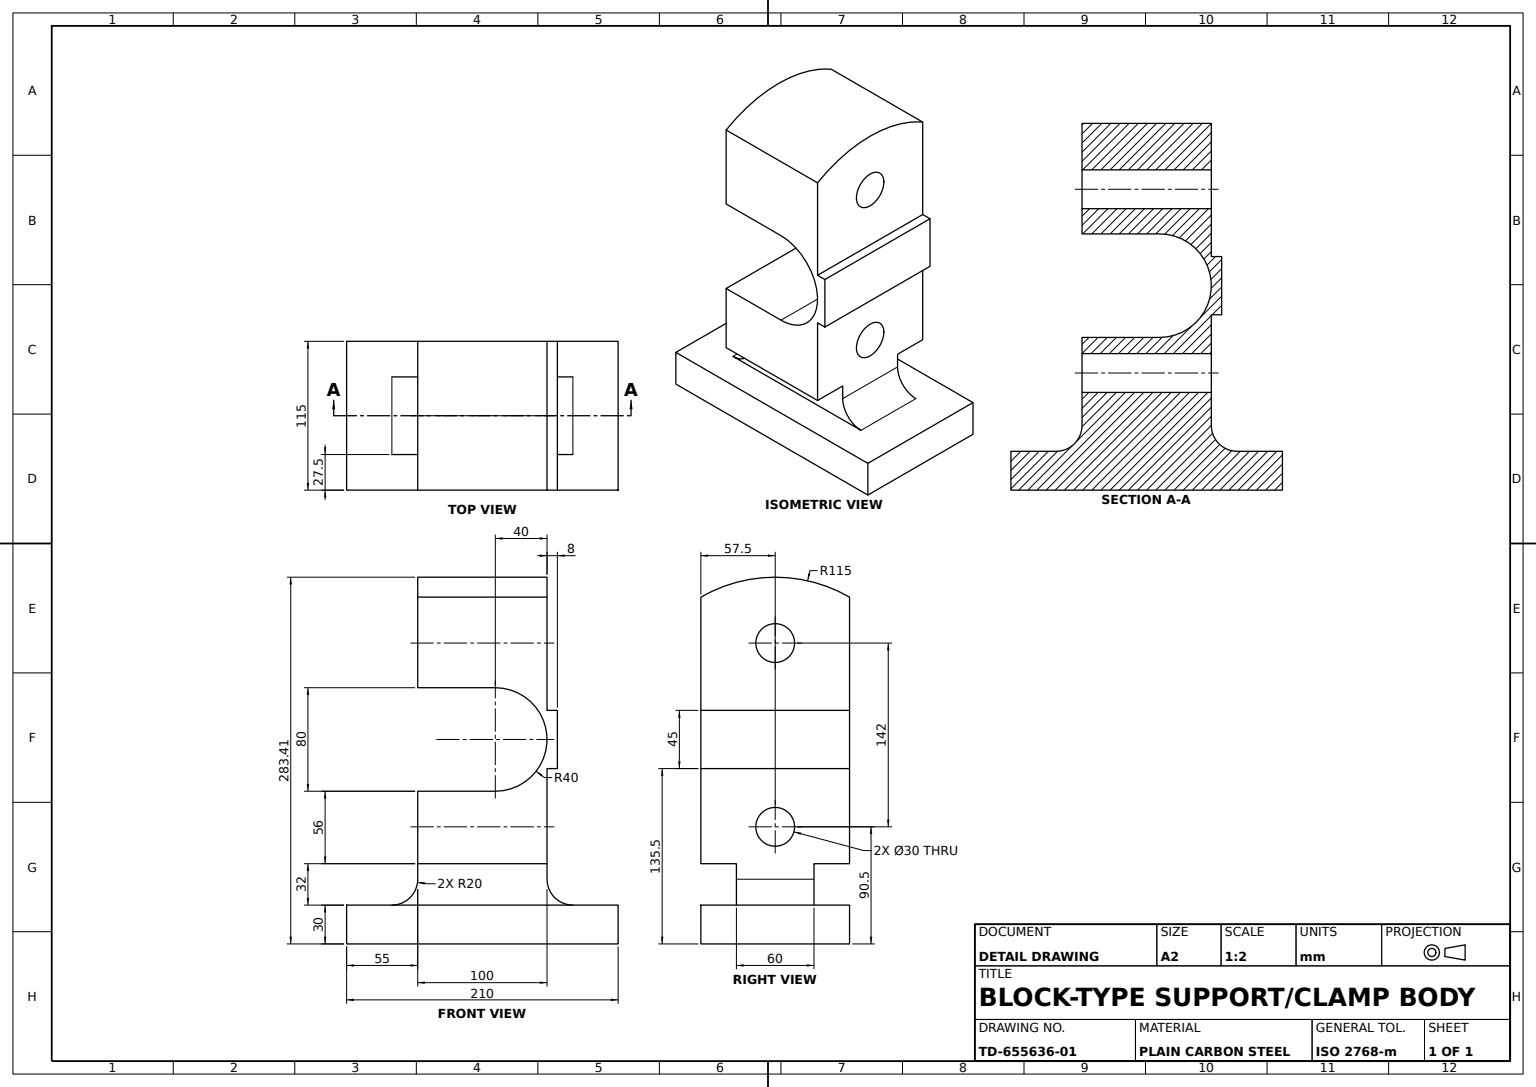
SolidWorks part; units mm, degrees
material "Plain Carbon Steel"
ref_plane "Front Plane" through (0, 0, 0) normal (0, 0, 1) x (1, 0, 0)
ref_plane "Top Plane" through (0, 0, 0) normal (0, 1, 0) x (1, 0, 0)
ref_plane "Right Plane" through (0, 0, 0) normal (1, 0, 0) x (0, 0, -1)
sketch "Base Plate Sketch" plane through (0, 0, 0) normal (0, 1, 0) x (1, 0, 0)
  line L1 (-105, -57.5) -> (105, -57.5)
  line L2 (-105, -57.5) -> (-105, 57.5)
  line L3 (-105, 57.5) -> (105, 57.5)
  line L4 (105, -57.5) -> (105, 57.5)
  line L5 (-105, -57.5) -> (105, 57.5) construction
  line L6 (-105, 57.5) -> (105, -57.5) construction
  point P0 (0, 0)
  dimension "D1" = 210
  dimension "D2" = 115
extrude "Base Plate 210x115x30" add sketch "Base Plate Sketch" along normal blind 30
sketch "Pedestal Sketch" plane through (0, 30, 0) normal (0, 1, 0) x (1, 0, 0)
  line L1 (-50, -30) -> (50, -30)
  line L2 (-50, -30) -> (-50, 30)
  line L3 (-50, 30) -> (50, 30)
  line L4 (50, -30) -> (50, 30)
  line L5 (-50, -30) -> (50, 30) construction
  line L6 (-50, 30) -> (50, -30) construction
  point P0 (0, 0)
  dimension "D1" = 100
  dimension "D2" = 60
extrude "Pedestal 100x60x32" add sketch "Pedestal Sketch" along normal blind 32
fillet "Pedestal Fillet R20" radius 20 2 edges at (50, 30, 0) (-50, 30, 0)
ref_plane "Plane1" through (0, 0, 0) normal (0, 0, 1) x (1, 0, 0)
sketch "Clamp Block Profile Sketch" plane through (0, 0, 0) normal (0, 0, 1) x (1, 0, 0)
  line L0 (50, 62) -> (50, 118)
  line L1 (50, 118) -> (50, 135.5)
  line L2 (50, 135.5) -> (58, 135.5)
  line L3 (58, 135.5) -> (58, 180.5)
  line L4 (58, 180.5) -> (50, 180.5)
  line L5 (50, 180.5) -> (50, 198)
  line L6 (50, 198) -> (50, 268)
  line L7 (50, 268) -> (-50, 268)
  line L8 (-50, 268) -> (-50, 198)
  line L9 (-50, 198) -> (10, 198)
  line L11 (10, 118) -> (-50, 118)
  line L12 (-50, 118) -> (-50, 62)
  line L13 (-50, 62) -> (50, 62)
  arc A1 (10, 118) -> (10, 198) centre (10, 158) ccw
  dimension "D1" = 56
  dimension "D3" = 40
  dimension "D2" = 60
  dimension "D4" = 100
  dimension "D5" = 45
  dimension "D6" = 8
  dimension "D7" = 110
  dimension "D8" = 48
  dimension "D9" = 22.5
extrude "Clamp Block" add sketch "Clamp Block Profile Sketch" along normal mid plane 115
sketch "Cross Holes Sketch" plane through (-50, 0, 0) normal (-1, 0, 0) x (0, 0, 1)
  line L0 (57.5, 118) -> (-57.5, 118) construction
  line L1 (57.5, 198) -> (-57.5, 198) construction
  circle A0 centre (0, 90.5) radius 15
  circle A1 centre (0, 232.5) radius 15
  dimension "D1" = 30
  dimension "D2" = 30
  dimension "D3" = 27.5
  dimension "D4" = 90.5
  dimension "D5" = 142
  dimension "D6" = 34.5
extrude "Cross Holes 2xØ30" cut sketch "Cross Holes Sketch" against normal blind 115
sketch "Clamp Band Sketch" plane through (-50, 0, 0) normal (-1, 0, 0) x (0, 0, 1)
  line L0 (-57.5, 268) -> (57.5, 268)
  arc A0 (-57.5, 268) -> (57.5, 268) centre (0, 168.4071) cw
extrude "Clamp Band" add sketch "Clamp Band Sketch" against normal blind 100
